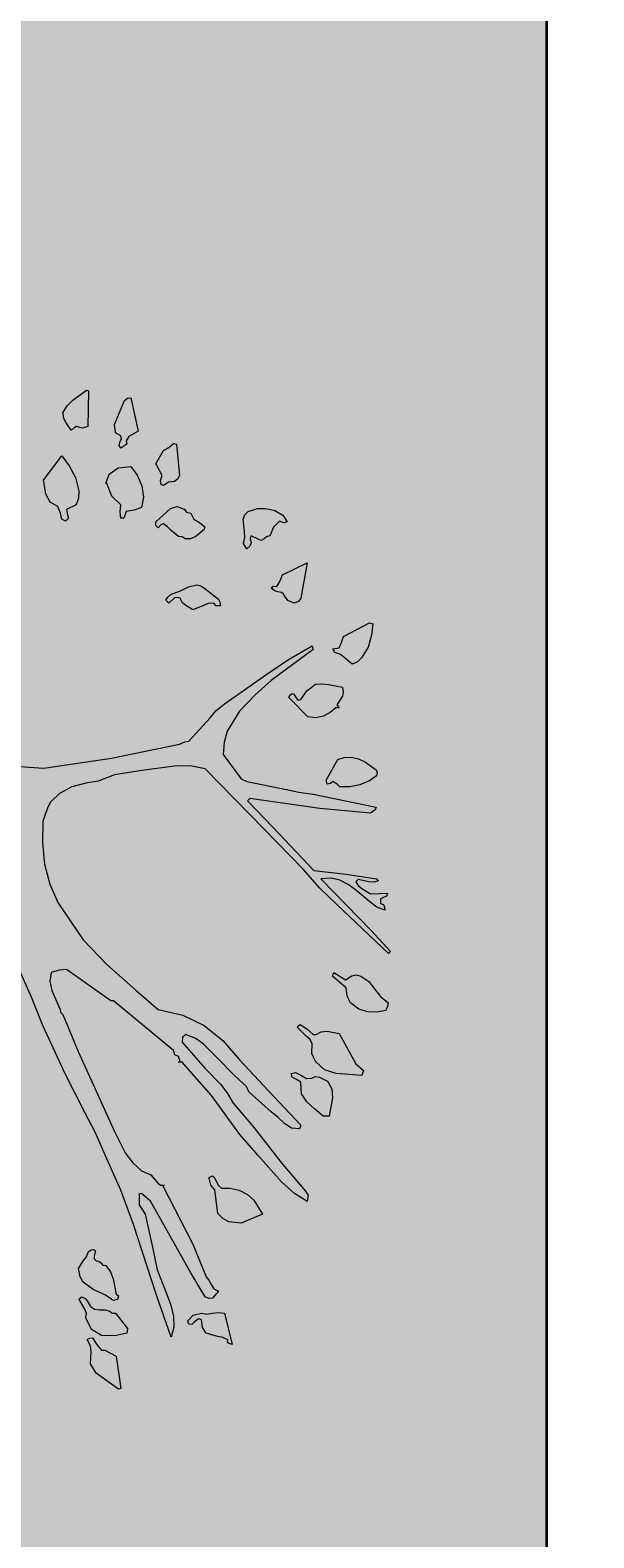
# Model space of a CAD drawing. Units: inches. Extents: x 84 to 1044, y -280 to 906.
# Tile 100 of 105: x 885 to 897, y 445 to 478. Entities that reach past the tile are written whole.
import ezdxf

# ---------------------------------------------------------------- set-up
doc = ezdxf.new("R2010")
doc.units = ezdxf.units.IN
for name, color, linetype, lineweight in [('A-ANNO-DIMS', 2, 'Continuous', 18), ('L-PLNT', 114, 'Continuous', 15), ('WALL', 250, 'Continuous', 35)]:
    doc.layers.add(name, color=color, linetype=linetype, lineweight=lineweight)
doc.layers.add('L-PLNT-PATT', color=9, linetype='Continuous', lineweight=9, true_color=0xafd9aa)
doc.styles.get("Standard").update_dxf_attribs({"font": 'arial.ttf'})
doc.dimstyles.get("Standard").update_dxf_attribs({"dimtxt": 0.18, "dimasz": 0.18, "dimexe": 0.18, "dimexo": 0.0625, "dimgap": 0.09, "dimtad": 0, "dimtih": 1, "dimtoh": 1, "dimdec": 4, "dimzin": 0, "dimdsep": 46, "dimtxsty": 'Standard', "dimcen": 0.09, "dimadec": 0, "dimazin": 0, "dimtfac": 1, "dimtdec": 4, "dimtofl": 0, "dimtmove": 0, "dimatfit": 3, "dimfxl": 1, "dimtolj": 1, "dimtzin": 0, "dimarcsym": 0})

# ---------------------------------------------------------------- blocks, each defined once
blk = doc.blocks.new('A$C37E508DF')
for p, q in [((0.9686, 1.4334), (0.9875, 1.4476)), ((0.9875, 1.4476), (0.9905, 1.4467)), ((0.9905, 1.4467), (0.9896, 1.3966)), ((0.9545, 1.4159), (0.9605, 1.4257)), ((0.9605, 1.4257), (0.9686, 1.4334)), ((1.0269, 1.3996), (1.0411, 1.433)), ((1.0411, 1.433), (1.045, 1.4365)), ((1.045, 1.4365), (1.0497, 1.4369)), ((1.0497, 1.4369), (1.0604, 1.3901)), ((0.9549, 1.4146), (0.9545, 1.4159)), ((0.9558, 1.4077), (0.9549, 1.4146)), ((0.9592, 1.4017), (0.9558, 1.4077)), ((0.966, 1.3914), (0.9592, 1.4017)), ((1.0282, 1.3876), (1.0269, 1.3996)), ((0.9703, 1.3944), (0.966, 1.3914)), ((0.9733, 1.3966), (0.9703, 1.3944)), ((0.9819, 1.3944), (0.9733, 1.3966)), ((0.9896, 1.3966), (0.9819, 1.3944)), ((1.0359, 1.3833), (1.0282, 1.3876)), ((1.0334, 1.37), (1.0351, 1.376)), ((1.0351, 1.376), (1.0368, 1.3794)), ((1.0368, 1.3794), (1.0359, 1.3833)), ((1.0471, 1.3824), (1.0432, 1.3764)), ((1.0432, 1.3764), (1.0441, 1.3717)), ((1.0604, 1.3901), (1.0471, 1.3824)), ((0.9274, 1.3215), (0.9532, 1.3554)), ((0.9532, 1.3554), (0.9635, 1.3413)), ((1.0359, 1.3661), (1.0334, 1.37)), ((1.0441, 1.3717), (1.0359, 1.3661)), ((1.0848, 1.3443), (1.0955, 1.3631)), ((1.0955, 1.3631), (1.1033, 1.367)), ((1.1033, 1.367), (1.1097, 1.373)), ((1.1097, 1.373), (1.114, 1.3717)), ((1.114, 1.3717), (1.1183, 1.328)), ((0.9635, 1.3413), (0.9721, 1.325)), ((1.0197, 1.3297), (1.0321, 1.3387)), ((1.0321, 1.3387), (1.0497, 1.3404)), ((1.0497, 1.3404), (1.0587, 1.3284)), ((1.0861, 1.343), (1.0848, 1.3443)), ((1.0938, 1.328), (1.0861, 1.343)), ((0.9279, 1.3194), (0.9274, 1.3215)), ((0.9305, 1.3018), (0.9279, 1.3194)), ((0.9721, 1.325), (0.9768, 1.3061)), ((1.0149, 1.3172), (1.0171, 1.3232)), ((1.0162, 1.3164), (1.0149, 1.3172)), ((1.0231, 1.2988), (1.0162, 1.3164)), ((1.0171, 1.3232), (1.0197, 1.3297)), ((1.0587, 1.3284), (1.0651, 1.3134)), ((1.0651, 1.3134), (1.0677, 1.2975)), ((1.0917, 1.3207), (1.0938, 1.328)), ((1.0925, 1.3151), (1.0917, 1.3207)), ((1.0955, 1.3138), (1.0925, 1.3151)), ((1.1028, 1.3185), (1.0955, 1.3138)), ((1.111, 1.3194), (1.1028, 1.3185)), ((1.1153, 1.3228), (1.111, 1.3194)), ((1.1183, 1.328), (1.1153, 1.3228)), ((0.9365, 1.2902), (0.9305, 1.3018)), ((0.9763, 1.2962), (0.9733, 1.2868)), ((0.9768, 1.3061), (0.9763, 1.2962)), ((1.0359, 1.2868), (1.0231, 1.2988)), ((1.0677, 1.2975), (1.0647, 1.2829)), ((0.9476, 1.2842), (0.9365, 1.2902)), ((0.951, 1.2748), (0.9476, 1.2842)), ((0.9532, 1.2666), (0.951, 1.2748)), ((0.9733, 1.2868), (0.9596, 1.2799)), ((0.9596, 1.2799), (0.9605, 1.2744)), ((0.9605, 1.2744), (0.9626, 1.2679)), ((1.0347, 1.2769), (1.0359, 1.2868)), ((1.0359, 1.2679), (1.0347, 1.2769)), ((1.0432, 1.2774), (1.0402, 1.2679)), ((1.0544, 1.2791), (1.0432, 1.2774)), ((1.0647, 1.2829), (1.0544, 1.2791)), ((1.0848, 1.2628), (1.1054, 1.2817)), ((1.1054, 1.2817), (1.1148, 1.2842)), ((1.1148, 1.2842), (1.1247, 1.2804)), ((1.1247, 1.2804), (1.1281, 1.2765)), ((1.1281, 1.2765), (1.1341, 1.2752)), ((1.1341, 1.2752), (1.1384, 1.2666)), ((1.2075, 1.2666), (1.21, 1.2726)), ((1.21, 1.2726), (1.2147, 1.2774)), ((1.2147, 1.2774), (1.2276, 1.2817)), ((1.2276, 1.2817), (1.2392, 1.2817)), ((1.2392, 1.2817), (1.2521, 1.2787)), ((1.2521, 1.2787), (1.2632, 1.2722)), ((1.2632, 1.2722), (1.2692, 1.2628)), ((0.9583, 1.2636), (0.9532, 1.2666)), ((0.9626, 1.2679), (0.9583, 1.2636)), ((1.0402, 1.2679), (1.0359, 1.2679)), ((1.0852, 1.2576), (1.0848, 1.2628)), ((1.0883, 1.2546), (1.0852, 1.2576)), ((1.0921, 1.2585), (1.0883, 1.2546)), ((1.0955, 1.2602), (1.0921, 1.2585)), ((1.1015, 1.2559), (1.0955, 1.2602)), ((1.1063, 1.2508), (1.1015, 1.2559)), ((1.117, 1.2422), (1.1063, 1.2508)), ((1.1384, 1.2666), (1.1461, 1.2619)), ((1.1526, 1.2521), (1.141, 1.2422)), ((1.1461, 1.2619), (1.1539, 1.2559)), ((1.1539, 1.2559), (1.1526, 1.2521)), ((1.2096, 1.2491), (1.2075, 1.2666)), ((1.21, 1.2409), (1.2096, 1.2491)), ((1.2503, 1.2551), (1.2448, 1.2431)), ((1.2585, 1.2636), (1.2503, 1.2551)), ((1.2645, 1.2615), (1.2585, 1.2636)), ((1.2692, 1.2628), (1.2645, 1.2615)), ((1.1221, 1.2418), (1.117, 1.2422)), ((1.126, 1.2388), (1.1221, 1.2418)), ((1.1337, 1.2388), (1.126, 1.2388)), ((1.141, 1.2422), (1.1337, 1.2388)), ((1.2079, 1.2323), (1.21, 1.2409)), ((1.2126, 1.2251), (1.2079, 1.2323)), ((1.2169, 1.2285), (1.2126, 1.2251)), ((1.2186, 1.2332), (1.2169, 1.2285)), ((1.2186, 1.2431), (1.2173, 1.2392)), ((1.2173, 1.2392), (1.2186, 1.2332)), ((1.2285, 1.2383), (1.2186, 1.2431)), ((1.2328, 1.2366), (1.2285, 1.2383)), ((1.2371, 1.2388), (1.2328, 1.2366)), ((1.2405, 1.2418), (1.2371, 1.2388)), ((1.2448, 1.2431), (1.2405, 1.2418)), ((1.2589, 1.1792), (1.2628, 1.1882)), ((1.2628, 1.1882), (1.2975, 1.2053)), ((1.2975, 1.2053), (1.2885, 1.1556)), ((1.1063, 1.1612), (1.1187, 1.1655)), ((1.1187, 1.1655), (1.1307, 1.1714)), ((1.1307, 1.1714), (1.1423, 1.1744)), ((1.1423, 1.1744), (1.1483, 1.1732)), ((1.1483, 1.1732), (1.1539, 1.1693)), ((1.1539, 1.1693), (1.1727, 1.1543)), ((1.2469, 1.1702), (1.2495, 1.1723)), ((1.2478, 1.1693), (1.2469, 1.1702)), ((1.2516, 1.1659), (1.2478, 1.1693)), ((1.2495, 1.1723), (1.2546, 1.1719)), ((1.2563, 1.1646), (1.2516, 1.1659)), ((1.2546, 1.1719), (1.2589, 1.1792)), ((1.2611, 1.1637), (1.2563, 1.1646)), ((1.099, 1.153), (1.102, 1.1573)), ((1.1033, 1.1487), (1.099, 1.153)), ((1.102, 1.1573), (1.1063, 1.1612)), ((1.111, 1.156), (1.1033, 1.1487)), ((1.1153, 1.1564), (1.111, 1.156)), ((1.1191, 1.1556), (1.1153, 1.1564)), ((1.1226, 1.1492), (1.1191, 1.1556)), ((1.1273, 1.1453), (1.1226, 1.1492)), ((1.1367, 1.1393), (1.1273, 1.1453)), ((1.1517, 1.1453), (1.1367, 1.1393)), ((1.1586, 1.1483), (1.1517, 1.1453)), ((1.1663, 1.1487), (1.1586, 1.1483)), ((1.1697, 1.1449), (1.1663, 1.1487)), ((1.1757, 1.1449), (1.1697, 1.1449)), ((1.1727, 1.1543), (1.1749, 1.1504)), ((1.1749, 1.1504), (1.1757, 1.1449)), ((1.2641, 1.1612), (1.2611, 1.1637)), ((1.2701, 1.1522), (1.2641, 1.1612)), ((1.2791, 1.1487), (1.2701, 1.1522)), ((1.2851, 1.1509), (1.2791, 1.1487)), ((1.2885, 1.1556), (1.2851, 1.1509)), ((1.3455, 1.0934), (1.3485, 1.102)), ((1.3485, 1.102), (1.385, 1.1209)), ((1.3875, 1.1037), (1.3828, 1.087)), ((1.385, 1.1209), (1.3897, 1.1196)), ((1.3897, 1.1196), (1.3875, 1.1037)), ((1.3057, 1.0835), (1.2469, 1.0402)), ((1.2713, 1.0694), (1.3044, 1.0887)), ((1.3044, 1.0887), (1.3057, 1.0835)), ((1.3335, 1.0844), (1.3421, 1.0861)), ((1.3361, 1.0793), (1.3335, 1.0844)), ((1.3421, 1.0861), (1.3455, 1.0934)), ((1.3828, 1.087), (1.3738, 1.072)), ((1.2409, 1.0488), (1.2713, 1.0694)), ((1.3434, 1.0771), (1.3361, 1.0793)), ((1.349, 1.0728), (1.3434, 1.0771)), ((1.3605, 1.063), (1.349, 1.0728)), ((1.3678, 1.0664), (1.3605, 1.063)), ((1.3738, 1.072), (1.3678, 1.0664)), ((1.1813, 1.0072), (1.2409, 1.0488)), ((1.2469, 1.0402), (1.2246, 1.0201)), ((1.2246, 1.0201), (1.2023, 0.9969)), ((1.2718, 1.0162), (1.2731, 1.0197)), ((1.2984, 0.9892), (1.2718, 1.0162)), ((1.2731, 1.0197), (1.2761, 1.0218)), ((1.2761, 1.0218), (1.2786, 1.0209)), ((1.2786, 1.0209), (1.2799, 1.0184)), ((1.2799, 1.0184), (1.2842, 1.0124)), ((1.2885, 1.0136), (1.2971, 1.0257)), ((1.2971, 1.0257), (1.3091, 1.0351)), ((1.3091, 1.0351), (1.3185, 1.0355)), ((1.3185, 1.0355), (1.3275, 1.0347)), ((1.3275, 1.0347), (1.3468, 1.0308)), ((1.3468, 1.018), (1.3391, 1.0059)), ((1.3468, 1.0308), (1.3481, 1.0239)), ((1.3481, 1.0239), (1.3468, 1.018)), ((1.1612, 0.9879), (1.1693, 0.9974)), ((1.1693, 0.9974), (1.1813, 1.0072)), ((1.2023, 0.9969), (1.1852, 0.9691)), ((1.2842, 1.0124), (1.2885, 1.0136)), ((1.3297, 0.9952), (1.3202, 0.9901)), ((1.3378, 1.0016), (1.3297, 0.9952)), ((1.3421, 1.0016), (1.3378, 1.0016)), ((1.3391, 1.0059), (1.3421, 1.0016)), ((1.1311, 0.9549), (1.1612, 0.9879)), ((1.3095, 0.9875), (1.2984, 0.9892)), ((1.3202, 0.9901), (1.3095, 0.9875)), ((1.1183, 0.9506), (1.1256, 0.954)), ((1.1256, 0.954), (1.1311, 0.9549)), ((1.1809, 0.9532), (1.1796, 0.936)), ((1.1852, 0.9691), (1.1809, 0.9532)), ((1.0227, 0.9309), (1.1183, 0.9506)), ((1.1796, 0.936), (1.2049, 0.9022)), ((1.3404, 0.9292), (1.3494, 0.9322)), ((1.3494, 0.9322), (1.3592, 0.9326)), ((1.3592, 0.9326), (1.3695, 0.93)), ((0.8936, 0.9193), (0.9279, 0.9172)), ((0.9279, 0.9172), (1.0227, 0.9309)), ((1.0685, 0.9142), (1.0269, 0.9077)), ((1.1114, 0.9198), (1.0685, 0.9142)), ((1.1333, 0.9202), (1.1114, 0.9198)), ((1.1543, 0.9159), (1.1333, 0.9202)), ((1.2371, 0.8314), (1.1543, 0.9159)), ((1.3241, 0.9), (1.3404, 0.9292)), ((1.3695, 0.93), (1.3794, 0.9253)), ((1.3794, 0.9253), (1.394, 0.9146)), ((1.394, 0.9146), (1.3957, 0.9112)), ((1.3957, 0.9112), (1.3948, 0.9065)), ((0.9673, 0.8906), (0.9498, 0.8816)), ((0.9866, 0.8962), (0.9673, 0.8906)), ((1.0042, 0.8987), (0.9866, 0.8962)), ((1.0269, 0.9077), (1.0042, 0.8987)), ((1.2049, 0.9022), (1.2126, 0.8983)), ((1.2126, 0.8983), (1.2662, 0.8876)), ((1.3254, 0.8944), (1.3241, 0.9)), ((1.3301, 0.8957), (1.3254, 0.8944)), ((1.3335, 0.8983), (1.3301, 0.8957)), ((1.3395, 0.8944), (1.3335, 0.8983)), ((1.3434, 0.8906), (1.3395, 0.8944)), ((1.3571, 0.8906), (1.3434, 0.8906)), ((1.3713, 0.8936), (1.3571, 0.8906)), ((1.3846, 0.8992), (1.3713, 0.8936)), ((1.3948, 0.9065), (1.3846, 0.8992)), ((0.9369, 0.8687), (0.933, 0.861)), ((0.9498, 0.8816), (0.9369, 0.8687)), ((1.2169, 0.8743), (1.2135, 0.8713)), ((1.2135, 0.8713), (1.2491, 0.834)), ((1.3151, 0.8606), (1.2169, 0.8743)), ((1.2662, 0.8876), (1.2855, 0.8833)), ((1.2855, 0.8833), (1.3057, 0.8807)), ((1.3057, 0.8807), (1.394, 0.8623)), ((0.9296, 0.852), (0.9262, 0.8421)), ((0.933, 0.861), (0.9296, 0.852)), ((1.3863, 0.8541), (1.3151, 0.8606)), ((1.3927, 0.8584), (1.3863, 0.8541)), ((1.394, 0.8623), (1.3927, 0.8584)), ((0.9262, 0.8421), (0.9257, 0.8121)), ((1.2919, 0.7752), (1.2371, 0.8314)), ((1.2491, 0.834), (1.3069, 0.7735)), ((0.9257, 0.8121), (0.9287, 0.7825)), ((0.9287, 0.7825), (0.936, 0.7542)), ((1.3151, 0.7487), (1.2919, 0.7752)), ((1.3069, 0.7735), (1.352, 0.7684)), ((1.3309, 0.7624), (1.3164, 0.7615)), ((1.3434, 0.7598), (1.3309, 0.7624)), ((1.352, 0.7684), (1.3948, 0.7615)), ((0.936, 0.7542), (0.9476, 0.7285)), ((1.3391, 0.7255), (1.3151, 0.7487)), ((1.3164, 0.7615), (1.3871, 0.6891)), ((1.355, 0.7538), (1.3434, 0.7598)), ((1.3653, 0.7461), (1.355, 0.7538)), ((1.3854, 0.7294), (1.3653, 0.7461)), ((1.3687, 0.7607), (1.3657, 0.7577)), ((1.3657, 0.7577), (1.3691, 0.7521)), ((1.3841, 0.7577), (1.3687, 0.7607)), ((1.3691, 0.7521), (1.3743, 0.7482)), ((1.3743, 0.7482), (1.3863, 0.7405)), ((1.3914, 0.7572), (1.3841, 0.7577)), ((1.3863, 0.7405), (1.4099, 0.7414)), ((1.397, 0.759), (1.3914, 0.7572)), ((1.3948, 0.7615), (1.397, 0.759)), ((1.4099, 0.7414), (1.4086, 0.7375)), ((0.9476, 0.7285), (0.9828, 0.6762)), ((1.4116, 0.6569), (1.3391, 0.7255)), ((1.3953, 0.7221), (1.3854, 0.7294)), ((1.4064, 0.7178), (1.3953, 0.7221)), ((1.4086, 0.7375), (1.4004, 0.7337)), ((1.4004, 0.7337), (1.4004, 0.7272)), ((1.4004, 0.7272), (1.4047, 0.7255)), ((1.4047, 0.7255), (1.406, 0.7221)), ((1.406, 0.7221), (1.4064, 0.7178)), ((1.3871, 0.6891), (1.4141, 0.6599)), ((0.9828, 0.6762), (1.0162, 0.6415)), ((1.4141, 0.6599), (1.4116, 0.6569)), ((1.0162, 0.6415), (1.0574, 0.605)), ((0.9103, 0.5956), (0.8932, 0.6342)), ((0.9382, 0.6303), (0.936, 0.6179)), ((0.936, 0.6179), (0.939, 0.605)), ((0.9493, 0.6333), (0.9382, 0.6303)), ((0.9596, 0.6342), (0.9493, 0.6333)), ((1.0218, 0.5904), (0.9596, 0.6342)), ((1.3327, 0.6252), (1.3348, 0.6303)), ((1.343, 0.6162), (1.3327, 0.6252)), ((1.3348, 0.6303), (1.3511, 0.62)), ((1.352, 0.6089), (1.343, 0.6162)), ((1.3511, 0.62), (1.3601, 0.6256)), ((1.3601, 0.6256), (1.3661, 0.6269)), ((1.3661, 0.6269), (1.3725, 0.6252)), ((1.3725, 0.6252), (1.3837, 0.6175)), ((1.3837, 0.6175), (1.3918, 0.6072)), ((0.9262, 0.5557), (0.9103, 0.5956)), ((0.939, 0.605), (0.9506, 0.5784)), ((1.0574, 0.605), (1.0883, 0.5784)), ((1.3533, 0.5969), (1.352, 0.6089)), ((1.358, 0.5874), (1.3533, 0.5969)), ((1.3918, 0.6072), (1.4004, 0.5964)), ((1.4004, 0.5964), (1.4111, 0.5874)), ((0.9506, 0.5784), (0.951, 0.5746)), ((0.951, 0.5746), (0.9545, 0.5711)), ((1.0256, 0.5904), (1.0218, 0.5904)), ((1.1097, 0.5205), (1.0256, 0.5904)), ((1.0883, 0.5784), (1.123, 0.5703)), ((1.37, 0.5789), (1.358, 0.5874)), ((1.3824, 0.575), (1.37, 0.5789)), ((1.3953, 0.5746), (1.3824, 0.575)), ((1.4077, 0.5771), (1.3953, 0.5746)), ((1.4103, 0.5823), (1.4077, 0.5771)), ((1.4111, 0.5874), (1.4103, 0.5823)), ((0.9583, 0.4871), (0.9262, 0.5557)), ((0.9545, 0.5711), (0.9759, 0.5193)), ((1.123, 0.5703), (1.1526, 0.5557)), ((1.1526, 0.5557), (1.1792, 0.5347)), ((1.2842, 0.554), (1.2855, 0.5557)), ((1.2842, 0.5527), (1.2842, 0.554)), ((1.2958, 0.5407), (1.2842, 0.5527)), ((1.2855, 0.5557), (1.2876, 0.557)), ((1.2876, 0.557), (1.2971, 0.551)), ((1.2971, 0.551), (1.3057, 0.5433)), ((1.1226, 0.5394), (1.1221, 0.5325)), ((1.1221, 0.5325), (1.1539, 0.4961)), ((1.1268, 0.5433), (1.1226, 0.5394)), ((1.141, 0.5377), (1.1268, 0.5433)), ((1.1521, 0.5296), (1.141, 0.5377)), ((1.1706, 0.5111), (1.1521, 0.5296)), ((1.1792, 0.5347), (1.2027, 0.5072)), ((1.3014, 0.536), (1.2958, 0.5407)), ((1.3044, 0.53), (1.3014, 0.536)), ((1.3039, 0.5167), (1.3044, 0.53)), ((1.3057, 0.5433), (1.3099, 0.5433)), ((1.3099, 0.5433), (1.3172, 0.5467)), ((1.3172, 0.5467), (1.3254, 0.548)), ((1.3254, 0.548), (1.3421, 0.5446)), ((1.3421, 0.5446), (1.3657, 0.5021)), ((0.9759, 0.5193), (1.0269, 0.4069)), ((1.1118, 0.5145), (1.1097, 0.5205)), ((1.117, 0.5124), (1.1118, 0.5145)), ((1.1191, 0.5055), (1.117, 0.5124)), ((1.1955, 0.4858), (1.1706, 0.5111)), ((1.3091, 0.5055), (1.3039, 0.5167)), ((0.9853, 0.4335), (0.9583, 0.4871)), ((1.117, 0.5042), (1.1191, 0.5055)), ((1.1217, 0.5042), (1.117, 0.5042)), ((1.1633, 0.4575), (1.1217, 0.5042)), ((1.1539, 0.4961), (1.1762, 0.4729)), ((1.2027, 0.5072), (1.2426, 0.4644)), ((1.2748, 0.4884), (1.2812, 0.4897)), ((1.2761, 0.4832), (1.2748, 0.4884)), ((1.2812, 0.4897), (1.2885, 0.4862)), ((1.3215, 0.4935), (1.3091, 0.5055)), ((1.3382, 0.4884), (1.3215, 0.4935)), ((1.3743, 0.4858), (1.3382, 0.4884)), ((1.3657, 0.5021), (1.3764, 0.4927)), ((1.3764, 0.4927), (1.3743, 0.4858)), ((1.1762, 0.4729), (1.1856, 0.4605)), ((1.207, 0.4747), (1.1955, 0.4858)), ((1.2122, 0.47), (1.207, 0.4747)), ((1.2156, 0.4627), (1.2122, 0.47)), ((1.2825, 0.4798), (1.2761, 0.4832)), ((1.2885, 0.4764), (1.2825, 0.4798)), ((1.2885, 0.4862), (1.2962, 0.4815)), ((1.2894, 0.4601), (1.2885, 0.4764)), ((1.2962, 0.4815), (1.3039, 0.482)), ((1.3039, 0.482), (1.3087, 0.4841)), ((1.3087, 0.4841), (1.3147, 0.4832)), ((1.3147, 0.4832), (1.3258, 0.4777)), ((1.3258, 0.4777), (1.3318, 0.4669)), ((1.3318, 0.4669), (1.3331, 0.4545)), ((1.2027, 0.4026), (1.1633, 0.4575)), ((1.1856, 0.4605), (1.1933, 0.4468)), ((1.1933, 0.4468), (1.2212, 0.4146)), ((1.2469, 0.4348), (1.2156, 0.4627)), ((1.2426, 0.4644), (1.2885, 0.4159)), ((1.2967, 0.4485), (1.2894, 0.4601)), ((1.3082, 0.4386), (1.2967, 0.4485)), ((1.3331, 0.4545), (1.3284, 0.4284)), ((1.0003, 0.4052), (0.9853, 0.4335)), ((1.2568, 0.4266), (1.2469, 0.4348)), ((1.2658, 0.4176), (1.2568, 0.4266)), ((1.3198, 0.4284), (1.3082, 0.4386)), ((1.3284, 0.4284), (1.3198, 0.4284)), ((1.0145, 0.373), (1.0003, 0.4052)), ((1.0269, 0.4069), (1.0419, 0.3769)), ((1.2289, 0.373), (1.2027, 0.4026)), ((1.2212, 0.4146), (1.2628, 0.361)), ((1.2752, 0.4116), (1.2658, 0.4176)), ((1.2868, 0.4108), (1.2752, 0.4116)), ((1.2885, 0.4159), (1.2868, 0.4108)), ((1.0359, 0.3246), (1.0145, 0.373)), ((1.0419, 0.3769), (1.0527, 0.3632)), ((1.0527, 0.3632), (1.0647, 0.352)), ((1.2615, 0.3362), (1.2289, 0.373)), ((1.2628, 0.361), (1.2949, 0.3233)), ((1.0647, 0.352), (1.078, 0.346)), ((1.078, 0.346), (1.0883, 0.334)), ((1.1599, 0.3426), (1.1646, 0.3447)), ((1.1599, 0.3413), (1.1599, 0.3426)), ((1.162, 0.3319), (1.1599, 0.3413)), ((1.1646, 0.3447), (1.168, 0.3417)), ((1.168, 0.3417), (1.1702, 0.3366)), ((1.0535, 0.2766), (1.0359, 0.3246)), ((1.0647, 0.3199), (1.0617, 0.3194)), ((1.0617, 0.3194), (1.0617, 0.304)), ((1.0711, 0.3147), (1.0647, 0.3199)), ((1.0883, 0.334), (1.0921, 0.3319)), ((1.0921, 0.3319), (1.0968, 0.3319)), ((1.0968, 0.3319), (1.0947, 0.3306)), ((1.0947, 0.3306), (1.1367, 0.2491)), ((1.1676, 0.325), (1.162, 0.3319)), ((1.1719, 0.292), (1.1676, 0.325)), ((1.1702, 0.3366), (1.1727, 0.3314)), ((1.1727, 0.3314), (1.177, 0.3276)), ((1.177, 0.3276), (1.1895, 0.3276)), ((1.1895, 0.3276), (1.2019, 0.3246)), ((1.2019, 0.3246), (1.2135, 0.3186)), ((1.2135, 0.3186), (1.2225, 0.3104)), ((1.2795, 0.3199), (1.2615, 0.3362)), ((1.2975, 0.3087), (1.2795, 0.3199)), ((1.2949, 0.3233), (1.2988, 0.3173)), ((1.0617, 0.304), (1.0698, 0.2911)), ((1.0775, 0.3092), (1.0711, 0.3147)), ((1.1341, 0.2084), (1.0775, 0.3092)), ((1.2225, 0.3104), (1.2349, 0.2911)), ((1.2988, 0.3173), (1.2975, 0.3087)), ((1.0861, 0.1775), (1.0535, 0.2766)), ((1.0698, 0.2911), (1.0805, 0.2448)), ((1.1792, 0.2847), (1.1719, 0.292)), ((1.1873, 0.28), (1.1792, 0.2847)), ((1.2049, 0.2783), (1.1873, 0.28)), ((1.2349, 0.2911), (1.2049, 0.2783)), ((0.9879, 0.2311), (0.9905, 0.2384)), ((0.9905, 0.2384), (0.9943, 0.241)), ((0.9943, 0.241), (0.9973, 0.2414)), ((0.9973, 0.2414), (1.0003, 0.2393)), ((1.0003, 0.2393), (0.9986, 0.232)), ((1.0805, 0.2448), (1.087, 0.2127)), ((1.1367, 0.2491), (1.1556, 0.2032)), ((0.9759, 0.214), (0.9836, 0.226)), ((0.9768, 0.2127), (0.9759, 0.214)), ((0.9789, 0.2028), (0.9768, 0.2127)), ((0.9836, 0.226), (0.9879, 0.2311)), ((0.9986, 0.232), (0.9986, 0.2281)), ((0.9986, 0.2281), (1.0012, 0.2255)), ((1.0012, 0.2255), (1.0051, 0.2251)), ((1.0051, 0.2251), (1.0076, 0.2225)), ((1.0076, 0.2225), (1.0106, 0.2195)), ((1.0106, 0.2195), (1.0149, 0.2191)), ((1.0149, 0.2191), (1.0214, 0.2101)), ((1.087, 0.2127), (1.0998, 0.1797)), ((0.9832, 0.1955), (0.9789, 0.2028)), ((0.9969, 0.1852), (0.9832, 0.1955)), ((1.0214, 0.2101), (1.0252, 0.2002)), ((1.0252, 0.2002), (1.0295, 0.1788)), ((1.1543, 0.1749), (1.1341, 0.2084)), ((1.1556, 0.2032), (1.1594, 0.1985)), ((1.1594, 0.1985), (1.1624, 0.1921)), ((1.1624, 0.1921), (1.1663, 0.1861)), ((0.9768, 0.1719), (0.9811, 0.1749)), ((0.9776, 0.1711), (0.9768, 0.1719)), ((0.9853, 0.1578), (0.9776, 0.1711)), ((0.9811, 0.1749), (0.9858, 0.1728)), ((0.9858, 0.1728), (0.9884, 0.1694)), ((0.9884, 0.1694), (0.9931, 0.1616)), ((1.0132, 0.1779), (0.9969, 0.1852)), ((1.0256, 0.1698), (1.0132, 0.1779)), ((1.0312, 0.1711), (1.0256, 0.1698)), ((1.0295, 0.1788), (1.0325, 0.1762)), ((1.0325, 0.1762), (1.0312, 0.1711)), ((1.1063, 0.1183), (1.0861, 0.1775)), ((1.0998, 0.1797), (1.1058, 0.1634)), ((1.1594, 0.1728), (1.1543, 0.1749)), ((1.1646, 0.1732), (1.1594, 0.1728)), ((1.1727, 0.1827), (1.1646, 0.1732)), ((1.1663, 0.1861), (1.1727, 0.1827)), ((0.9879, 0.1518), (0.9853, 0.1578)), ((0.9866, 0.1453), (0.9879, 0.1518)), ((0.9931, 0.1616), (0.9991, 0.1574)), ((0.9991, 0.1574), (1.0059, 0.1565)), ((1.0059, 0.1565), (1.0132, 0.1565)), ((1.0132, 0.1565), (1.0205, 0.1548)), ((1.0205, 0.1548), (1.0235, 0.1522)), ((1.0235, 0.1522), (1.0282, 0.1518)), ((1.0282, 0.1518), (1.0454, 0.1303)), ((1.1058, 0.1634), (1.1097, 0.1475)), ((1.1298, 0.1411), (1.1376, 0.1492)), ((1.1376, 0.1492), (1.1491, 0.1518)), ((1.1491, 0.1518), (1.1564, 0.1505)), ((1.1564, 0.1505), (1.1642, 0.1518)), ((1.1642, 0.1518), (1.1727, 0.1531)), ((1.1727, 0.1531), (1.1813, 0.1518)), ((1.1813, 0.1518), (1.192, 0.108)), ((0.9948, 0.1291), (0.9866, 0.1453)), ((1.0089, 0.1205), (0.9948, 0.1291)), ((1.0454, 0.1303), (1.0441, 0.1239)), ((1.1101, 0.1325), (1.1063, 0.1183)), ((1.1097, 0.1475), (1.1101, 0.1325)), ((1.1311, 0.1364), (1.1298, 0.1411)), ((1.1354, 0.1359), (1.1311, 0.1364)), ((1.1384, 0.1389), (1.1354, 0.1359)), ((1.1423, 0.1423), (1.1384, 0.1389)), ((1.1449, 0.1441), (1.1423, 0.1423)), ((1.1491, 0.1428), (1.1449, 0.1441)), ((1.1504, 0.132), (1.1491, 0.1428)), ((1.1556, 0.1239), (1.1504, 0.132)), ((0.9884, 0.1149), (0.9918, 0.117)), ((0.9935, 0.1063), (0.9884, 0.1149)), ((0.9918, 0.117), (0.9961, 0.1175)), ((0.9943, 0.0982), (0.9935, 0.1063)), ((0.9961, 0.1175), (1.0016, 0.1085)), ((1.0016, 0.1085), (1.0089, 0.0999)), ((1.0274, 0.12), (1.0089, 0.1205)), ((1.0441, 0.1239), (1.0274, 0.12)), ((1.1714, 0.1192), (1.1556, 0.1239)), ((1.1792, 0.1179), (1.1714, 0.1192)), ((1.186, 0.1145), (1.1792, 0.1179)), ((1.1856, 0.111), (1.186, 0.1145)), ((1.1873, 0.1093), (1.1856, 0.111)), ((1.192, 0.108), (1.1873, 0.1093)), ((0.9931, 0.081), (0.9943, 0.0982)), ((1.0089, 0.0999), (1.0132, 0.0999)), ((1.0132, 0.0999), (1.0295, 0.0917)), ((1.0295, 0.0917), (1.0359, 0.0463)), ((1.0012, 0.0677), (0.9931, 0.081)), ((1.0325, 0.0454), (1.0012, 0.0677)), ((1.0359, 0.0463), (1.0325, 0.0454))]:
    blk.add_line(p, q)
blk = doc.blocks.new('*D62')
at = {"layer": 'A-ANNO-DIMS', "color": 0, "lineweight": -2, "transparency": 16777216}
for p, q in [((203.179, 709.183), (203.179, 905.9)), ((203.359, 905.72), (549.232, 905.72)), ((895.894, 905.72), (550.021, 905.72)), ((896.074, 400.183), (896.074, 905.9))]:
    blk.add_line(p, q, dxfattribs=at)
at = {"layer": 'A-ANNO-DIMS', "color": 0, "transparency": 16777216}
for points in [[(203.359, 905.75), (203.359, 905.69), (203.179, 905.72)], [(895.894, 905.75), (895.894, 905.69), (896.074, 905.72)]]:
    blk.add_solid(points, dxfattribs=at)
at = {"layer": 'Defpoints', "color": 0, "transparency": 16777216}
for p in [(896.074, 905.72), (203.179, 709.12), (896.074, 400.12)]:
    blk.add_point(p, dxfattribs=at)
at = {"layer": 'A-ANNO-DIMS', "color": 0, "transparency": 16777216, "insert": (549.627, 905.72), "char_height": 0.18, "attachment_point": 5}
blk.add_mtext('\\A1;692.9', dxfattribs=at)
blk = doc.blocks.new('*D63')
at = {"layer": 'A-ANNO-DIMS', "color": 0, "lineweight": -2, "transparency": 16777216}
for p, q in [((833.136, 709.12), (1043.768, 709.12)), ((1043.588, 708.94), (1043.588, 400.302)), ((1043.588, 91.3), (1043.588, 399.938)), ((896.136, 91.12), (1043.768, 91.12))]:
    blk.add_line(p, q, dxfattribs=at)
at = {"layer": 'A-ANNO-DIMS', "color": 0, "transparency": 16777216}
for points in [[(1043.558, 708.94), (1043.618, 708.94), (1043.588, 709.12)], [(1043.558, 91.3), (1043.618, 91.3), (1043.588, 91.12)]]:
    blk.add_solid(points, dxfattribs=at)
at = {"layer": 'Defpoints', "color": 0, "transparency": 16777216}
for p in [(833.074, 709.12), (1043.588, 709.12), (896.074, 91.12)]:
    blk.add_point(p, dxfattribs=at)
at = {"layer": 'A-ANNO-DIMS', "color": 0, "transparency": 16777216, "insert": (1043.588, 400.12), "char_height": 0.18, "attachment_point": 5}
blk.add_mtext('\\A1;618', dxfattribs=at)
blk = doc.blocks.new('*D65')
at = {"layer": 'A-ANNO-DIMS', "color": 0, "lineweight": -2, "transparency": 16777216}
for p, q in [((896.074, 400.183), (896.074, 905.9)), ((896.254, 905.72), (943.855, 905.72)), ((991.894, 905.72), (944.293, 905.72)), ((992.074, 856.183), (992.074, 905.9))]:
    blk.add_line(p, q, dxfattribs=at)
at = {"layer": 'A-ANNO-DIMS', "color": 0, "transparency": 16777216}
for points in [[(896.254, 905.75), (896.254, 905.69), (896.074, 905.72)], [(991.894, 905.75), (991.894, 905.69), (992.074, 905.72)]]:
    blk.add_solid(points, dxfattribs=at)
at = {"layer": 'Defpoints', "color": 0, "transparency": 16777216}
for p in [(896.074, 905.72), (992.074, 856.12), (896.074, 400.12)]:
    blk.add_point(p, dxfattribs=at)
at = {"layer": 'A-ANNO-DIMS', "color": 0, "transparency": 16777216, "insert": (944.074, 905.72), "char_height": 0.18, "attachment_point": 5}
blk.add_mtext('\\A1;96', dxfattribs=at)

msp = doc.modelspace()

# ---------------------------------------------------------------- hatches: boundary and pattern name
at = {"layer": 'L-PLNT-PATT', "transparency": 33554597}
h = msp.add_hatch(color=256, dxfattribs=at)
h.dxf.hatch_style = 1
h.paths.add_polyline_path([(896.074, 511.12), (704.074, 511.12), (704.074, 491.62), (704.074, 419.62), (704.074, 400.12), (833.074, 400.12), (896.074, 400.12)])

# ---------------------------------------------------------------- linework, layer by layer
at = {"layer": 'WALL'}
msp.add_line((896.074, 400.12), (896.074, 511.12), dxfattribs=at)

# ---------------------------------------------------------------- block references
at = {"layer": 'L-PLNT', "xscale": 15.19586232982809, "yscale": 15.19586232982809, "zscale": 15.19586232982809}
msp.add_blockref('A$C37E508DF', (871.246, 447.963), dxfattribs=at)

# ---------------------------------------------------------------- dimensions: what is measured, and where the dimension line sits
at = {"layer": 'A-ANNO-DIMS'}
for p1, override, picture, middle in [((203.179, 709.12), {"dimdec": 1, "dimlfac": 1, "dimrnd": 0, "dimzin": 0, "dimdsep": 46, "dimlunit": 2}, '*D62', (549.627, 905.72)), ((992.074, 856.12), {"dimdec": 0, "dimlfac": 1, "dimrnd": 0, "dimzin": 0, "dimdsep": 46, "dimlunit": 2}, '*D65', (944.074, 905.72))]:
    dim = msp.add_linear_dim(base=(896.074, 905.72), p1=p1, p2=(896.074, 400.12), dimstyle='Standard', override=override, dxfattribs=at)
    dim.commit()
    dim.dimension.update_dxf_attribs({"geometry": picture, "text_midpoint": middle})
dim = msp.add_linear_dim(base=(1043.588, 709.12), p1=(896.074, 91.12), p2=(833.074, 709.12), angle=90, dimstyle='Standard', override={"dimdec": 0, "dimlfac": 1, "dimrnd": 0, "dimzin": 0, "dimdsep": 46, "dimlunit": 2}, dxfattribs=at)
dim.commit()
dim.dimension.update_dxf_attribs({"geometry": '*D63', "text_midpoint": (1043.588, 400.12)})

doc.saveas('drawing.dxf')
